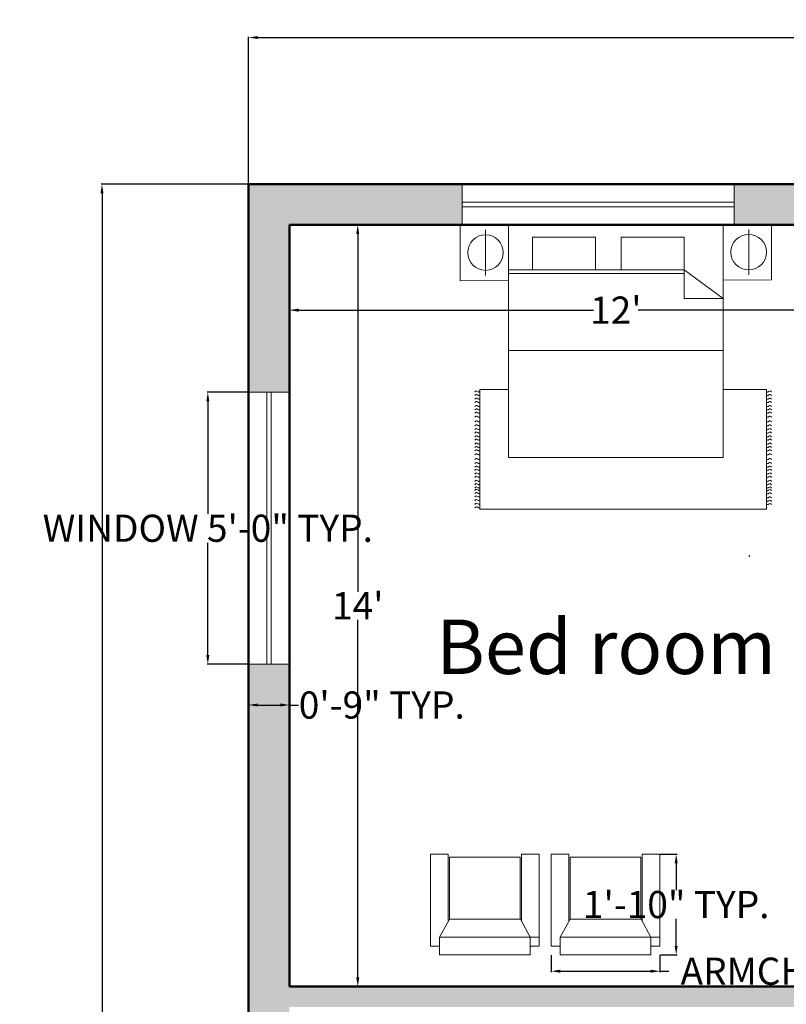
# Model space of a CAD drawing. Units: inches. Extents: x 2436 to 2989, y 5527 to 6207.
# Tile 3 of 5: x 2436 to 2605, y 5989 to 6207. Entities that reach past the tile are written whole.
import ezdxf

# ---------------------------------------------------------------- set-up
doc = ezdxf.new("R2010")
doc.units = ezdxf.units.IN
doc.header["$MEASUREMENT"] = 0
for name, color, linetype, lineweight in [('A-ANNO-DIMS', 2, 'Continuous', 18), ('A-AREA-IDEN', 7, 'Continuous', 25), ('A-FURN', 8, 'Continuous', 18), ('A-GLAZ', 4, 'Continuous', 18), ('A-WALL', 7, 'Continuous', 50), ('A-WALL-PATT', 252, 'Continuous', 13)]:
    doc.layers.add(name, color=color, linetype=linetype, lineweight=lineweight)
doc.styles.get("Standard").update_dxf_attribs({"font": 'arial.ttf'})
doc.dimstyles.get("Standard").update_dxf_attribs({"dimtxt": 6, "dimasz": 2, "dimexe": 0.18, "dimexo": 0.0625, "dimgap": 0.09, "dimtad": 0, "dimtih": 1, "dimtoh": 1, "dimdec": 0, "dimzin": 0, "dimdsep": 46, "dimlunit": 3, "dimtxsty": 'Standard', "dimcen": 0.09, "dimadec": 0, "dimazin": 0, "dimtfac": 1, "dimtdec": 0, "dimtofl": 0, "dimtmove": 0, "dimatfit": 3, "dimfxl": 1, "dimtolj": 1, "dimtzin": 0, "dimarcsym": 0})

# ---------------------------------------------------------------- blocks, each defined once
blk = doc.blocks.new('*D3')
at = {"layer": 'A-ANNO-DIMS', "color": 0, "lineweight": -2, "transparency": 16777216}
for p, q in [((2495.45, 6161.23), (2510.64, 6161.23)), ((2510.46, 6159.23), (2510.46, 6080.33)), ((2510.46, 5995.23), (2510.46, 6074.13)), ((2495.45, 5993.23), (2510.64, 5993.23))]:
    blk.add_line(p, q, dxfattribs=at)
at = {"layer": 'A-ANNO-DIMS', "color": 0, "transparency": 16777216}
for points in [[(2510.12, 6159.23), (2510.79, 6159.23), (2510.46, 6161.23)], [(2510.12, 5995.23), (2510.79, 5995.23), (2510.46, 5993.23)]]:
    blk.add_solid(points, dxfattribs=at)
at = {"layer": 'Defpoints', "color": 0, "transparency": 16777216}
for p in [(2495.39, 6161.23), (2495.39, 5993.23), (2510.46, 5993.23)]:
    blk.add_point(p, dxfattribs=at)
at = {"layer": 'A-ANNO-DIMS', "color": 0, "transparency": 16777216, "insert": (2510.46, 6077.23), "char_height": 6, "attachment_point": 5}
blk.add_mtext("\\A1;14'", dxfattribs=at)
blk = doc.blocks.new('*D4')
at = {"layer": 'A-ANNO-DIMS', "color": 0, "lineweight": -2, "transparency": 16777216}
for p, q in [((2495.39, 6161.17), (2495.39, 6142.26)), ((2639.39, 6161.17), (2639.39, 6142.26)), ((2497.39, 6142.44), (2562.49, 6142.44)), ((2637.39, 6142.44), (2572.29, 6142.44))]:
    blk.add_line(p, q, dxfattribs=at)
at = {"layer": 'A-ANNO-DIMS', "color": 0, "transparency": 16777216}
for points in [[(2497.39, 6142.77), (2497.39, 6142.1), (2495.39, 6142.44)], [(2637.39, 6142.77), (2637.39, 6142.1), (2639.39, 6142.44)]]:
    blk.add_solid(points, dxfattribs=at)
at = {"layer": 'Defpoints', "color": 0, "transparency": 16777216}
for p in [(2495.39, 6161.23), (2639.39, 6161.23), (2639.39, 6142.44)]:
    blk.add_point(p, dxfattribs=at)
at = {"layer": 'A-ANNO-DIMS', "color": 0, "transparency": 16777216, "insert": (2567.39, 6142.44), "char_height": 6, "attachment_point": 5}
blk.add_mtext("\\A1;12'", dxfattribs=at)
blk = doc.blocks.new('BED-WITH-NIGHTSTANDS')
for p, q in [((5.6, 61.62), (5.6, 51.56)), ((63.65, 61.72), (63.65, 51.66)), ((49.39, 52.82), (10.63, 52.82)), ((49.39, 52.82), (58, 46.47)), ((49.44, 52.82), (49.44, 46.47)), ((49.44, 52), (10.63, 52)), ((49.44, 46.47), (58, 46.47)), ((58.05, 34.96), (10.63, 34.96)), ((4.35, 0), (4.35, 26.37)), ((4.35, 26.37), (10.65, 26.37)), ((58.05, 26.37), (67.59, 26.37)), ((67.59, 26.37), (67.59, 0)), ((4.35, 0), (67.59, 0))]:
    blk.add_line(p, q)
for points in [[(0, 50.39), (10.63, 50.5), (10.63, 62.68), (0, 62.58)], [(58.05, 62.68), (58.05, 11.37), (10.63, 11.37), (10.63, 62.68)], [(58.05, 50.5), (68.68, 50.6), (68.68, 62.78), (58.05, 62.68)], [(29.88, 59.98), (29.88, 52.82), (15.98, 52.82), (15.98, 59.98)], [(49.44, 59.98), (49.44, 52.82), (35.55, 52.82), (35.55, 59.98)]]:
    blk.add_lwpolyline(points, close=True)
for centre in [(5.6, 56.59), (63.65, 56.69)]:
    blk.add_circle(centre, 3.92)
for points, knots in [([(3.23, 25.84), (3.32, 25.96), (3.52, 26.2), (3.86, 25.96), (4.14, 25.78), (4.29, 25.89), (4.35, 25.94)], [0, 0, 0, 0, 0.400747, 0.791423, 1.067667, 1.29709, 1.29709, 1.29709, 1.29709]), ([(68.71, 25.84), (68.61, 25.96), (68.42, 26.2), (68.08, 25.96), (67.8, 25.78), (67.65, 25.89), (67.58, 25.94)], [0, 0, 0, 0, 0.400747, 0.791423, 1.067667, 1.29709, 1.29709, 1.29709, 1.29709]), ([(3.23, 25.06), (3.32, 25.18), (3.52, 25.42), (3.86, 25.18), (4.14, 25.01), (4.29, 25.11), (4.35, 25.16)], [0, 0, 0, 0, 0.400747, 0.791423, 1.067667, 1.29709, 1.29709, 1.29709, 1.29709]), ([(3.23, 24.24), (3.32, 24.36), (3.52, 24.6), (3.86, 24.36), (4.14, 24.19), (4.29, 24.3), (4.35, 24.34)], [0, 0, 0, 0, 0.400747, 0.791423, 1.067667, 1.29709, 1.29709, 1.29709, 1.29709]), ([(68.71, 25.06), (68.61, 25.18), (68.42, 25.42), (68.08, 25.18), (67.8, 25.01), (67.65, 25.11), (67.58, 25.16)], [0, 0, 0, 0, 0.400747, 0.791423, 1.067667, 1.29709, 1.29709, 1.29709, 1.29709]), ([(68.71, 24.24), (68.61, 24.36), (68.42, 24.6), (68.08, 24.36), (67.8, 24.19), (67.65, 24.3), (67.58, 24.34)], [0, 0, 0, 0, 0.400747, 0.791423, 1.067667, 1.29709, 1.29709, 1.29709, 1.29709]), ([(3.23, 23.51), (3.32, 23.63), (3.52, 23.87), (3.86, 23.63), (4.14, 23.46), (4.29, 23.57), (4.35, 23.62)], [0, 0, 0, 0, 0.400747, 0.791423, 1.067667, 1.29709, 1.29709, 1.29709, 1.29709]), ([(3.23, 22.63), (3.32, 22.75), (3.52, 22.99), (3.86, 22.75), (4.14, 22.58), (4.29, 22.69), (4.35, 22.73)], [0, 0, 0, 0, 0.400747, 0.791423, 1.067667, 1.29709, 1.29709, 1.29709, 1.29709]), ([(3.23, 21.88), (3.32, 22), (3.52, 22.24), (3.86, 22), (4.14, 21.83), (4.29, 21.93), (4.35, 21.98)], [0, 0, 0, 0, 0.400747, 0.791423, 1.067667, 1.29709, 1.29709, 1.29709, 1.29709]), ([(68.71, 23.51), (68.61, 23.63), (68.42, 23.87), (68.08, 23.63), (67.8, 23.46), (67.65, 23.57), (67.58, 23.62)], [0, 0, 0, 0, 0.400747, 0.791423, 1.067667, 1.29709, 1.29709, 1.29709, 1.29709]), ([(68.71, 22.63), (68.61, 22.75), (68.42, 22.99), (68.08, 22.75), (67.8, 22.58), (67.65, 22.69), (67.58, 22.73)], [0, 0, 0, 0, 0.400747, 0.791423, 1.067667, 1.29709, 1.29709, 1.29709, 1.29709]), ([(68.71, 21.88), (68.61, 22), (68.42, 22.24), (68.08, 22), (67.8, 21.83), (67.65, 21.93), (67.58, 21.98)], [0, 0, 0, 0, 0.400747, 0.791423, 1.067667, 1.29709, 1.29709, 1.29709, 1.29709]), ([(3.23, 21.15), (3.32, 21.27), (3.52, 21.51), (3.86, 21.27), (4.14, 21.1), (4.29, 21.21), (4.35, 21.25)], [0, 0, 0, 0, 0.400747, 0.791423, 1.067667, 1.29709, 1.29709, 1.29709, 1.29709]), ([(3.23, 20.27), (3.32, 20.39), (3.52, 20.63), (3.86, 20.39), (4.14, 20.22), (4.29, 20.32), (4.35, 20.37)], [0, 0, 0, 0, 0.400747, 0.791423, 1.067667, 1.29709, 1.29709, 1.29709, 1.29709]), ([(68.71, 21.15), (68.61, 21.27), (68.42, 21.51), (68.08, 21.27), (67.8, 21.1), (67.65, 21.21), (67.58, 21.25)], [0, 0, 0, 0, 0.400747, 0.791423, 1.067667, 1.29709, 1.29709, 1.29709, 1.29709]), ([(68.71, 20.27), (68.61, 20.39), (68.42, 20.63), (68.08, 20.39), (67.8, 20.22), (67.65, 20.32), (67.58, 20.37)], [0, 0, 0, 0, 0.400747, 0.791423, 1.067667, 1.29709, 1.29709, 1.29709, 1.29709]), ([(3.23, 19.23), (3.32, 19.35), (3.52, 19.59), (3.86, 19.35), (4.14, 19.18), (4.29, 19.29), (4.35, 19.33)], [0, 0, 0, 0, 0.400747, 0.791423, 1.067667, 1.29709, 1.29709, 1.29709, 1.29709]), ([(3.23, 18.35), (3.32, 18.47), (3.52, 18.71), (3.86, 18.47), (4.14, 18.3), (4.29, 18.4), (4.35, 18.45)], [0, 0, 0, 0, 0.400747, 0.791423, 1.067667, 1.29709, 1.29709, 1.29709, 1.29709]), ([(3.23, 17.53), (3.32, 17.65), (3.52, 17.89), (3.86, 17.65), (4.14, 17.48), (4.29, 17.59), (4.35, 17.64)], [0, 0, 0, 0, 0.400747, 0.791423, 1.067667, 1.29709, 1.29709, 1.29709, 1.29709]), ([(68.71, 19.23), (68.61, 19.35), (68.42, 19.59), (68.08, 19.35), (67.8, 19.18), (67.65, 19.29), (67.58, 19.33)], [0, 0, 0, 0, 0.400747, 0.791423, 1.067667, 1.29709, 1.29709, 1.29709, 1.29709]), ([(68.71, 18.35), (68.61, 18.47), (68.42, 18.71), (68.08, 18.47), (67.8, 18.3), (67.65, 18.4), (67.58, 18.45)], [0, 0, 0, 0, 0.400747, 0.791423, 1.067667, 1.29709, 1.29709, 1.29709, 1.29709]), ([(68.71, 17.53), (68.61, 17.65), (68.42, 17.89), (68.08, 17.65), (67.8, 17.48), (67.65, 17.59), (67.58, 17.64)], [0, 0, 0, 0, 0.400747, 0.791423, 1.067667, 1.29709, 1.29709, 1.29709, 1.29709]), ([(3.23, 16.76), (3.32, 16.88), (3.52, 17.12), (3.86, 16.88), (4.14, 16.71), (4.29, 16.81), (4.35, 16.86)], [0, 0, 0, 0, 0.400747, 0.791423, 1.067667, 1.29709, 1.29709, 1.29709, 1.29709]), ([(3.23, 15.94), (3.32, 16.06), (3.52, 16.3), (3.86, 16.06), (4.14, 15.89), (4.29, 16), (4.35, 16.04)], [0, 0, 0, 0, 0.400747, 0.791423, 1.067667, 1.29709, 1.29709, 1.29709, 1.29709]), ([(3.23, 15.21), (3.32, 15.33), (3.52, 15.57), (3.86, 15.33), (4.14, 15.16), (4.29, 15.27), (4.35, 15.32)], [0, 0, 0, 0, 0.400747, 0.791423, 1.067667, 1.29709, 1.29709, 1.29709, 1.29709]), ([(68.71, 16.76), (68.61, 16.88), (68.42, 17.12), (68.08, 16.88), (67.8, 16.71), (67.65, 16.81), (67.58, 16.86)], [0, 0, 0, 0, 0.400747, 0.791423, 1.067667, 1.29709, 1.29709, 1.29709, 1.29709]), ([(68.71, 15.94), (68.61, 16.06), (68.42, 16.3), (68.08, 16.06), (67.8, 15.89), (67.65, 16), (67.58, 16.04)], [0, 0, 0, 0, 0.400747, 0.791423, 1.067667, 1.29709, 1.29709, 1.29709, 1.29709]), ([(68.71, 15.21), (68.61, 15.33), (68.42, 15.57), (68.08, 15.33), (67.8, 15.16), (67.65, 15.27), (67.58, 15.32)], [0, 0, 0, 0, 0.400747, 0.791423, 1.067667, 1.29709, 1.29709, 1.29709, 1.29709]), ([(3.23, 14.33), (3.32, 14.45), (3.52, 14.69), (3.86, 14.45), (4.14, 14.28), (4.29, 14.39), (4.35, 14.43)], [0, 0, 0, 0, 0.400747, 0.791423, 1.067667, 1.29709, 1.29709, 1.29709, 1.29709]), ([(3.23, 13.58), (3.32, 13.7), (3.52, 13.94), (3.86, 13.7), (4.14, 13.53), (4.29, 13.63), (4.35, 13.68)], [0, 0, 0, 0, 0.400747, 0.791423, 1.067667, 1.29709, 1.29709, 1.29709, 1.29709]), ([(3.23, 12.85), (3.32, 12.97), (3.52, 13.21), (3.86, 12.97), (4.14, 12.8), (4.29, 12.9), (4.35, 12.95)], [0, 0, 0, 0, 0.400747, 0.791423, 1.067667, 1.29709, 1.29709, 1.29709, 1.29709]), ([(68.71, 14.33), (68.61, 14.45), (68.42, 14.69), (68.08, 14.45), (67.8, 14.28), (67.65, 14.39), (67.58, 14.43)], [0, 0, 0, 0, 0.400747, 0.791423, 1.067667, 1.29709, 1.29709, 1.29709, 1.29709]), ([(68.71, 13.58), (68.61, 13.7), (68.42, 13.94), (68.08, 13.7), (67.8, 13.53), (67.65, 13.63), (67.58, 13.68)], [0, 0, 0, 0, 0.400747, 0.791423, 1.067667, 1.29709, 1.29709, 1.29709, 1.29709]), ([(68.71, 12.85), (68.61, 12.97), (68.42, 13.21), (68.08, 12.97), (67.8, 12.8), (67.65, 12.9), (67.58, 12.95)], [0, 0, 0, 0, 0.400747, 0.791423, 1.067667, 1.29709, 1.29709, 1.29709, 1.29709]), ([(3.23, 11.97), (3.32, 12.09), (3.52, 12.33), (3.86, 12.09), (4.14, 11.92), (4.29, 12.02), (4.35, 12.07)], [0, 0, 0, 0, 0.400747, 0.791423, 1.067667, 1.29709, 1.29709, 1.29709, 1.29709]), ([(3.23, 10.93), (3.32, 11.05), (3.52, 11.29), (3.86, 11.05), (4.14, 10.88), (4.29, 10.99), (4.35, 11.03)], [0, 0, 0, 0, 0.400747, 0.791423, 1.067667, 1.29709, 1.29709, 1.29709, 1.29709]), ([(68.71, 11.97), (68.61, 12.09), (68.42, 12.33), (68.08, 12.09), (67.8, 11.92), (67.65, 12.02), (67.58, 12.07)], [0, 0, 0, 0, 0.400747, 0.791423, 1.067667, 1.29709, 1.29709, 1.29709, 1.29709]), ([(68.71, 10.93), (68.61, 11.05), (68.42, 11.29), (68.08, 11.05), (67.8, 10.88), (67.65, 10.99), (67.58, 11.03)], [0, 0, 0, 0, 0.400747, 0.791423, 1.067667, 1.29709, 1.29709, 1.29709, 1.29709]), ([(3.23, 10.05), (3.32, 10.17), (3.52, 10.41), (3.86, 10.17), (4.14, 10), (4.29, 10.1), (4.35, 10.15)], [0, 0, 0, 0, 0.400747, 0.791423, 1.067667, 1.29709, 1.29709, 1.29709, 1.29709]), ([(3.23, 9.23), (3.32, 9.35), (3.52, 9.59), (3.86, 9.35), (4.14, 9.18), (4.29, 9.29), (4.35, 9.34)], [0, 0, 0, 0, 0.400747, 0.791423, 1.067667, 1.29709, 1.29709, 1.29709, 1.29709]), ([(3.23, 8.54), (3.32, 8.66), (3.52, 8.9), (3.86, 8.66), (4.14, 8.49), (4.29, 8.6), (4.35, 8.65)], [0, 0, 0, 0, 0.400747, 0.791423, 1.067667, 1.29709, 1.29709, 1.29709, 1.29709]), ([(68.71, 10.05), (68.61, 10.17), (68.42, 10.41), (68.08, 10.17), (67.8, 10), (67.65, 10.1), (67.58, 10.15)], [0, 0, 0, 0, 0.400747, 0.791423, 1.067667, 1.29709, 1.29709, 1.29709, 1.29709]), ([(68.71, 9.23), (68.61, 9.35), (68.42, 9.59), (68.08, 9.35), (67.8, 9.18), (67.65, 9.29), (67.58, 9.34)], [0, 0, 0, 0, 0.400747, 0.791423, 1.067667, 1.29709, 1.29709, 1.29709, 1.29709]), ([(68.71, 8.54), (68.61, 8.66), (68.42, 8.9), (68.08, 8.66), (67.8, 8.49), (67.65, 8.6), (67.58, 8.65)], [0, 0, 0, 0, 0.400747, 0.791423, 1.067667, 1.29709, 1.29709, 1.29709, 1.29709]), ([(3.23, 7.73), (3.32, 7.85), (3.52, 8.09), (3.86, 7.85), (4.14, 7.68), (4.29, 7.78), (4.35, 7.83)], [0, 0, 0, 0, 0.400747, 0.791423, 1.067667, 1.29709, 1.29709, 1.29709, 1.29709]), ([(3.23, 7), (3.32, 7.12), (3.52, 7.36), (3.86, 7.12), (4.14, 6.95), (4.29, 7.05), (4.35, 7.1)], [0, 0, 0, 0, 0.400747, 0.791423, 1.067667, 1.29709, 1.29709, 1.29709, 1.29709]), ([(68.71, 7.73), (68.61, 7.85), (68.42, 8.09), (68.08, 7.85), (67.8, 7.68), (67.65, 7.78), (67.58, 7.83)], [0, 0, 0, 0, 0.400747, 0.791423, 1.067667, 1.29709, 1.29709, 1.29709, 1.29709]), ([(68.71, 7), (68.61, 7.12), (68.42, 7.36), (68.08, 7.12), (67.8, 6.95), (67.65, 7.05), (67.58, 7.1)], [0, 0, 0, 0, 0.400747, 0.791423, 1.067667, 1.29709, 1.29709, 1.29709, 1.29709]), ([(3.23, 6.12), (3.32, 6.24), (3.52, 6.48), (3.86, 6.24), (4.14, 6.07), (4.29, 6.17), (4.35, 6.22)], [0, 0, 0, 0, 0.400747, 0.791423, 1.067667, 1.29709, 1.29709, 1.29709, 1.29709]), ([(3.23, 5.36), (3.32, 5.49), (3.52, 5.73), (3.86, 5.49), (4.14, 5.31), (4.29, 5.42), (4.35, 5.47)], [0, 0, 0, 0, 0.400747, 0.791423, 1.067667, 1.29709, 1.29709, 1.29709, 1.29709]), ([(3.23, 4.64), (3.32, 4.76), (3.52, 5), (3.86, 4.76), (4.14, 4.59), (4.29, 4.69), (4.35, 4.74)], [0, 0, 0, 0, 0.400747, 0.791423, 1.067667, 1.29709, 1.29709, 1.29709, 1.29709]), ([(3.23, 4.13), (3.32, 4.25), (3.52, 4.49), (3.86, 4.25), (4.14, 4.08), (4.29, 4.18), (4.35, 4.23)], [0, 0, 0, 0, 0.400747, 0.791423, 1.067667, 1.29709, 1.29709, 1.29709, 1.29709]), ([(68.71, 6.12), (68.61, 6.24), (68.42, 6.48), (68.08, 6.24), (67.8, 6.07), (67.65, 6.17), (67.58, 6.22)], [0, 0, 0, 0, 0.400747, 0.791423, 1.067667, 1.29709, 1.29709, 1.29709, 1.29709]), ([(68.71, 5.36), (68.61, 5.49), (68.42, 5.73), (68.08, 5.49), (67.8, 5.31), (67.65, 5.42), (67.58, 5.47)], [0, 0, 0, 0, 0.400747, 0.791423, 1.067667, 1.29709, 1.29709, 1.29709, 1.29709]), ([(68.71, 4.64), (68.61, 4.76), (68.42, 5), (68.08, 4.76), (67.8, 4.59), (67.66, 4.69), (67.59, 4.73)], [0, 0, 0, 0, 0.400747, 0.791423, 1.067667, 1.283686, 1.283686, 1.283686, 1.283686]), ([(3.23, 3.44), (3.32, 3.56), (3.52, 3.8), (3.86, 3.56), (4.14, 3.39), (4.29, 3.49), (4.35, 3.54)], [0, 0, 0, 0, 0.400747, 0.791423, 1.067667, 1.29709, 1.29709, 1.29709, 1.29709]), ([(3.23, 2.67), (3.32, 2.79), (3.52, 3.03), (3.86, 2.79), (4.14, 2.62), (4.29, 2.73), (4.35, 2.78)], [0, 0, 0, 0, 0.400747, 0.791423, 1.067667, 1.29709, 1.29709, 1.29709, 1.29709]), ([(68.72, 4.07), (68.62, 4.19), (68.43, 4.43), (68.09, 4.19), (67.81, 4.01), (67.66, 4.12), (67.59, 4.17)], [0, 0, 0, 0, 0.400747, 0.791423, 1.067667, 1.29709, 1.29709, 1.29709, 1.29709]), ([(68.72, 3.34), (68.62, 3.46), (68.43, 3.7), (68.09, 3.46), (67.81, 3.29), (67.66, 3.39), (67.59, 3.44)], [0, 0, 0, 0, 0.400747, 0.791423, 1.067667, 1.29709, 1.29709, 1.29709, 1.29709]), ([(68.72, 2.46), (68.62, 2.58), (68.43, 2.82), (68.09, 2.58), (67.81, 2.4), (67.66, 2.51), (67.59, 2.56)], [0, 0, 0, 0, 0.400747, 0.791423, 1.067667, 1.29709, 1.29709, 1.29709, 1.29709]), ([(3.23, 1.86), (3.32, 1.98), (3.52, 2.22), (3.86, 1.98), (4.14, 1.81), (4.29, 1.92), (4.35, 1.97)], [0, 0, 0, 0, 0.400747, 0.791423, 1.067667, 1.29709, 1.29709, 1.29709, 1.29709]), ([(3.23, 1.05), (3.32, 1.17), (3.52, 1.41), (3.86, 1.17), (4.14, 1), (4.29, 1.11), (4.35, 1.15)], [0, 0, 0, 0, 0.400747, 0.791423, 1.067667, 1.29709, 1.29709, 1.29709, 1.29709]), ([(3.23, 0.28), (3.32, 0.4), (3.52, 0.64), (3.86, 0.4), (4.14, 0.22), (4.29, 0.33), (4.35, 0.38)], [0, 0, 0, 0, 0.400747, 0.791423, 1.067667, 1.29709, 1.29709, 1.29709, 1.29709]), ([(68.72, 1.7), (68.62, 1.82), (68.43, 2.06), (68.09, 1.82), (67.81, 1.65), (67.66, 1.76), (67.59, 1.81)], [0, 0, 0, 0, 0.400747, 0.791423, 1.067667, 1.29709, 1.29709, 1.29709, 1.29709]), ([(68.72, 0.98), (68.62, 1.1), (68.43, 1.34), (68.09, 1.1), (67.81, 0.93), (67.67, 1.03), (67.6, 1.07)], [0, 0, 0, 0, 0.400747, 0.791423, 1.067667, 1.283686, 1.283686, 1.283686, 1.283686])]:
    blk.add_open_spline(points, degree=3, knots=knots)
blk = doc.blocks.new('CHAIR-ARM')
for p, q in [((0, 1.96), (0, 22.23)), ((3.92, 22.23), (0, 22.23)), ((3.92, 7.54), (3.92, 22.23)), ((20.05, 7.41), (20.05, 22.23)), ((20.05, 22.23), (23.98, 22.23)), ((23.98, 1.96), (23.98, 22.23)), ((19.74, 21.58), (19.74, 7.85)), ((1.96, 3.92), (4.17, 7.85)), ((19.81, 7.85), (22.01, 3.92)), ((1.96, 3.92), (23.98, 3.92)), ((1.96, 3.92), (1.96, 0)), ((22.01, 3.92), (22.01, 0)), ((0, 1.96), (1.96, 1.96)), ((1.96, 0), (22.01, 0)), ((22.01, 1.96), (23.98, 1.96))]:
    blk.add_line(p, q)
blk.add_lwpolyline([(19.74, 21.58), (4.17, 21.58), (4.17, 7.85), (19.81, 7.85)])
blk = doc.blocks.new('WINDOW-60IN')
for p, q in [((0, 9), (0, 0)), ((60, 9), (0, 9)), ((60, 0), (60, 9)), ((60, 5), (0, 5)), ((0, 4), (60, 4)), ((0, 0), (60, 0))]:
    blk.add_line(p, q)
blk = doc.blocks.new('*D34')
at = {"layer": 'A-ANNO-DIMS', "color": 0, "lineweight": -2, "transparency": 16777216}
for p, q in [((2553.14, 6000.14), (2553.14, 5996.42)), ((2577.11, 6000.14), (2577.11, 5996.42)), ((2555.14, 5996.6), (2575.11, 5996.6)), ((2577.11, 5996.6), (2579.11, 5996.6))]:
    blk.add_line(p, q, dxfattribs=at)
at = {"layer": 'A-ANNO-DIMS', "color": 0, "transparency": 16777216}
for points in [[(2555.14, 5996.94), (2555.14, 5996.27), (2553.14, 5996.6)], [(2575.11, 5996.94), (2575.11, 5996.27), (2577.11, 5996.6)]]:
    blk.add_solid(points, dxfattribs=at)
at = {"layer": 'Defpoints', "color": 0, "transparency": 16777216}
for p in [(2553.14, 6000.2), (2577.11, 6000.2), (2577.11, 5996.6)]:
    blk.add_point(p, dxfattribs=at)
at = {"layer": 'A-ANNO-DIMS', "color": 0, "transparency": 16777216, "insert": (2621.18, 5996.6), "char_height": 6, "attachment_point": 5}
blk.add_mtext('\\A1;ARMCHAIR 2\'-0" TYP.', dxfattribs=at)
blk = doc.blocks.new('*D35')
at = {"layer": 'A-ANNO-DIMS', "color": 0, "lineweight": -2, "transparency": 16777216}
for p, q in [((2577.17, 6022.43), (2580.89, 6022.43)), ((2580.71, 6020.43), (2580.71, 6014.47)), ((2580.71, 6002.2), (2580.71, 6008.16)), ((2577.17, 6000.2), (2580.89, 6000.2))]:
    blk.add_line(p, q, dxfattribs=at)
at = {"layer": 'A-ANNO-DIMS', "color": 0, "transparency": 16777216}
for points in [[(2580.37, 6020.43), (2581.04, 6020.43), (2580.71, 6022.43)], [(2580.37, 6002.2), (2581.04, 6002.2), (2580.71, 6000.2)]]:
    blk.add_solid(points, dxfattribs=at)
at = {"layer": 'Defpoints', "color": 0, "transparency": 16777216}
for p in [(2577.11, 6022.43), (2580.71, 6022.43), (2577.11, 6000.2)]:
    blk.add_point(p, dxfattribs=at)
at = {"layer": 'A-ANNO-DIMS', "color": 0, "transparency": 16777216, "insert": (2580.71, 6011.31), "char_height": 6, "attachment_point": 5}
blk.add_mtext('\\A1;1\'-10" TYP.', dxfattribs=at)
blk = doc.blocks.new('*D38')
at = {"layer": 'A-ANNO-DIMS', "color": 0, "lineweight": -2, "transparency": 16777216}
for p, q in [((2486.33, 6124.33), (2477.21, 6124.33)), ((2477.39, 6122.33), (2477.39, 6097.53)), ((2477.39, 6066.33), (2477.39, 6091.14)), ((2486.33, 6064.33), (2477.21, 6064.33))]:
    blk.add_line(p, q, dxfattribs=at)
at = {"layer": 'A-ANNO-DIMS', "color": 0, "transparency": 16777216}
for points in [[(2477.05, 6122.33), (2477.72, 6122.33), (2477.39, 6124.33)], [(2477.05, 6066.33), (2477.72, 6066.33), (2477.39, 6064.33)]]:
    blk.add_solid(points, dxfattribs=at)
at = {"layer": 'Defpoints', "color": 0, "transparency": 16777216}
for p in [(2486.39, 6124.33), (2477.39, 6064.33), (2486.39, 6064.33)]:
    blk.add_point(p, dxfattribs=at)
at = {"layer": 'A-ANNO-DIMS', "color": 0, "transparency": 16777216, "insert": (2477.39, 6094.33), "char_height": 6, "attachment_point": 5}
blk.add_mtext('\\A1;WINDOW 5\'-0" TYP.', dxfattribs=at)
blk = doc.blocks.new('*D39')
at = {"layer": 'A-ANNO-DIMS', "color": 0, "lineweight": -2, "transparency": 16777216}
for p, q in [((2486.39, 6064.27), (2486.39, 6055.15)), ((2495.39, 6064.27), (2495.39, 6055.15)), ((2488.39, 6055.33), (2493.39, 6055.33)), ((2495.39, 6055.33), (2497.39, 6055.33))]:
    blk.add_line(p, q, dxfattribs=at)
at = {"layer": 'A-ANNO-DIMS', "color": 0, "transparency": 16777216}
for points in [[(2488.39, 6055.67), (2488.39, 6055), (2486.39, 6055.33)], [(2493.39, 6055.67), (2493.39, 6055), (2495.39, 6055.33)]]:
    blk.add_solid(points, dxfattribs=at)
at = {"layer": 'Defpoints', "color": 0, "transparency": 16777216}
for p in [(2486.39, 6064.33), (2495.39, 6064.33), (2495.39, 6055.33)]:
    blk.add_point(p, dxfattribs=at)
at = {"layer": 'A-ANNO-DIMS', "color": 0, "transparency": 16777216, "insert": (2515.76, 6055.33), "char_height": 6, "attachment_point": 5}
blk.add_mtext('\\A1;0\'-9" TYP.', dxfattribs=at)
blk = doc.blocks.new('*D48')
at = {"layer": 'A-ANNO-DIMS', "color": 0, "lineweight": -2, "transparency": 16777216}
for p, q in [((2486.39, 6170.29), (2486.39, 6202.76)), ((2488.39, 6202.58), (2705.49, 6202.58)), ((2943.39, 6202.58), (2726.28, 6202.58)), ((2945.39, 6080.73), (2945.39, 6202.76))]:
    blk.add_line(p, q, dxfattribs=at)
at = {"layer": 'A-ANNO-DIMS', "color": 0, "transparency": 16777216}
for points in [[(2488.39, 6202.92), (2488.39, 6202.25), (2486.39, 6202.58)], [(2943.39, 6202.92), (2943.39, 6202.25), (2945.39, 6202.58)]]:
    blk.add_solid(points, dxfattribs=at)
at = {"layer": 'Defpoints', "color": 0, "transparency": 16777216}
for p in [(2945.39, 6202.58), (2486.39, 6170.23), (2945.39, 6080.66)]:
    blk.add_point(p, dxfattribs=at)
at = {"layer": 'A-ANNO-DIMS', "color": 0, "transparency": 16777216, "insert": (2715.89, 6202.58), "char_height": 6, "attachment_point": 5}
blk.add_mtext('\\A1;38\'-3"', dxfattribs=at)
blk = doc.blocks.new('*D49')
at = {"layer": 'A-ANNO-DIMS', "color": 0, "lineweight": -2, "transparency": 16777216}
for p, q in [((2486.33, 6170.23), (2453.86, 6170.23)), ((2454.04, 6168.23), (2454.04, 5851.68)), ((2454.04, 5528.73), (2454.04, 5845.29)), ((2675.33, 5526.73), (2453.86, 5526.73))]:
    blk.add_line(p, q, dxfattribs=at)
at = {"layer": 'A-ANNO-DIMS', "color": 0, "transparency": 16777216}
for points in [[(2453.7, 6168.23), (2454.37, 6168.23), (2454.04, 6170.23)], [(2453.7, 5528.73), (2454.37, 5528.73), (2454.04, 5526.73)]]:
    blk.add_solid(points, dxfattribs=at)
at = {"layer": 'Defpoints', "color": 0, "transparency": 16777216}
for p in [(2486.39, 6170.23), (2454.04, 5526.73), (2675.39, 5526.73)]:
    blk.add_point(p, dxfattribs=at)
at = {"layer": 'A-ANNO-DIMS', "color": 0, "transparency": 16777216, "insert": (2454.04, 5848.48), "char_height": 6, "attachment_point": 5}
blk.add_mtext('\\A1;53\'-7 1/2"', dxfattribs=at)
blk = doc.blocks.new('*D56')
at = {"layer": 'A-ANNO-DIMS', "color": 0, "lineweight": -2, "transparency": 16777216}
for p, q in [((2596.78, 6088.19), (2596.96, 6088.19)), ((2596.87, 6088.1), (2596.87, 6088.28)), ((2699.31, 6088.19), (2662.89, 6088.19))]:
    blk.add_line(p, q, dxfattribs=at)
at = {"layer": 'A-ANNO-DIMS', "color": 0, "transparency": 16777216}
blk.add_solid([(2662.89, 6088.52), (2662.89, 6087.85), (2660.89, 6088.19)], dxfattribs=at)
at = {"layer": 'Defpoints', "color": 0, "transparency": 16777216}
for p in [(2596.87, 6088.19), (2660.89, 6088.19)]:
    blk.add_point(p, dxfattribs=at)
at = {"layer": 'A-ANNO-DIMS', "color": 0, "transparency": 16777216, "insert": (2716.81, 6088.19), "char_height": 6, "attachment_point": 5}
blk.add_mtext('\\A1;4X R5\'-4"', dxfattribs=at)

msp = doc.modelspace()

# ---------------------------------------------------------------- hatches: boundary and pattern name
at = {"layer": 'A-WALL-PATT'}
h = msp.add_hatch(color=256, dxfattribs=at)
h.dxf.hatch_style = 1
h.paths.add_polyline_path([(2533.49, 6170.23), (2486.39, 6170.23), (2486.39, 6124.33), (2495.39, 6124.33), (2495.39, 6161.23), (2533.49, 6161.23)])
h.paths.add_polyline_path([(2677.58, 6170.23), (2593.49, 6170.23), (2593.49, 6161.23), (2639.39, 6161.23), (2639.39, 6035.73), (2639.39, 6035.73), (2643.89, 6035.73), (2643.89, 6036.73), (2685.89, 6036.73), (2685.89, 6041.23), (2643.89, 6041.23), (2643.89, 6161.23), (2677.58, 6161.23)])
h.paths.add_polyline_path([(2792.39, 6170.23), (2737.58, 6170.23), (2737.58, 6161.23), (2787.89, 6161.23), (2787.89, 6084.23), (2792.39, 6084.23), (2792.39, 6161.23), (2936.39, 6161.23), (2936.39, 6071.23), (2840.39, 6071.23), (2840.39, 6047.23), (2792.39, 6047.23), (2792.39, 6048.23), (2787.89, 6048.23), (2787.89, 6047.23), (2787.89, 6041.23), (2742.3, 6041.23), (2742.3, 6036.73), (2787.89, 6036.73), (2787.89, 6035.73), (2792.39, 6035.73), (2792.39, 6042.73), (2840.39, 6042.73), (2840.39, 5945.23), (2792.39, 5945.23), (2792.39, 6003.73), (2787.89, 6003.73), (2787.89, 5893.73), (2792.39, 5893.73), (2792.39, 5940.73), (2845.89, 5940.73), (2845.89, 5945.23), (2844.89, 5945.23), (2844.89, 6047.23), (2844.89, 6066.73), (2936.39, 6066.73), (2936.39, 6024.33), (2945.39, 6024.33), (2945.39, 6080.66), (2940.89, 6080.66), (2940.89, 6165.73), (2792.39, 6165.73)])
h.paths.add_polyline_path([(2945.39, 6000.33), (2936.39, 6000.33), (2936.39, 5945.23), (2881.89, 5945.23), (2881.89, 5940.73), (2936.39, 5940.73), (2936.39, 5901.74), (2945.39, 5901.74)], flags=17)
h.paths.add_polyline_path([(2945.39, 5841.74), (2936.39, 5841.74), (2936.39, 5796.73), (2792.39, 5796.73), (2792.39, 5857.73), (2787.89, 5857.73), (2787.89, 5856.73), (2786.89, 5856.73), (2786.89, 5852.23), (2787.89, 5852.23), (2787.89, 5792.23), (2892.89, 5792.23), (2892.89, 5760.78), (2901.89, 5760.78), (2901.89, 5792.23), (2945.39, 5792.23)])
h.paths.add_polyline_path([(2495.39, 5880.74), (2486.39, 5880.74), (2486.39, 5787.73), (2525.39, 5787.73), (2525.39, 5761.57), (2534.39, 5761.57), (2534.39, 5792.23), (2639.39, 5792.23), (2639.39, 5733.23), (2643.89, 5733.23), (2643.89, 5852.23), (2750.89, 5852.23), (2750.89, 5856.73), (2643.89, 5856.73), (2643.89, 5857.73), (2639.39, 5857.73), (2639.39, 5796.73), (2495.39, 5796.73)])
h.paths.add_polyline_path([(2495.39, 6064.33), (2486.39, 6064.33), (2486.39, 5940.74), (2495.39, 5940.74), (2495.39, 5988.73), (2639.39, 5988.73), (2639.39, 5893.73), (2643.89, 5893.73), (2643.89, 5999.73), (2639.39, 5999.73), (2639.39, 5993.23), (2495.39, 5993.23)])
h.paths.add_polyline_path([(2682.14, 5696.23), (2643.89, 5696.23), (2643.89, 5697.23), (2639.39, 5697.23), (2639.39, 5696.23), (2558.39, 5696.23), (2534.39, 5696.23), (2534.39, 5737.57), (2525.39, 5737.57), (2525.39, 5687.23), (2534.39, 5687.23), (2558.39, 5687.23), (2643.89, 5687.23), (2682.14, 5687.23)])
h.paths.add_polyline_path([(2901.89, 5736.78), (2892.89, 5736.78), (2892.89, 5696.23), (2868.89, 5696.23), (2751.89, 5696.23), (2751.89, 5687.23), (2787.89, 5687.23), (2787.89, 5567.23), (2792.39, 5567.23), (2792.39, 5687.23), (2868.89, 5687.23), (2892.89, 5687.23), (2901.89, 5687.23)])
h.paths.add_polyline_path([(2643.89, 5687.23), (2639.39, 5687.23), (2639.39, 5567.23), (2643.89, 5567.23)])
h.paths.add_polyline_path([(2787.89, 5567.23), (2643.89, 5567.23), (2643.89, 5562.73), (2787.89, 5562.73)])
h.paths.add_polyline_path([(2643.89, 5567.23), (2639.39, 5567.23), (2639.39, 5562.73), (2643.89, 5562.73)])
h.paths.add_polyline_path([(2792.39, 5567.23), (2787.89, 5567.23), (2787.89, 5562.73), (2792.39, 5562.73)])

# ---------------------------------------------------------------- linework, layer by layer
at = {"layer": 'A-GLAZ'}
msp.add_line((2533.49, 6161.23), (2533.49, 6161.23), dxfattribs=at)
at = {"layer": 'A-WALL'}
for p, q in [((2486.39, 6170.23), (2792.39, 6170.23)), ((2486.39, 6170.23), (2486.39, 5787.73)), ((2495.39, 6161.23), (2639.39, 6161.23)), ((2495.39, 6161.23), (2495.39, 5993.23)), ((2495.39, 5993.23), (2639.39, 5993.23))]:
    msp.add_line(p, q, dxfattribs=at)

# ---------------------------------------------------------------- block references
at = {"layer": 'A-FURN'}
for name, p in [('BED-WITH-NIGHTSTANDS', (2533.05, 6098.55)), ('CHAIR-ARM', (2526.52, 6000.2)), ('CHAIR-ARM', (2553.14, 6000.2))]:
    msp.add_blockref(name, p, dxfattribs=at)
at = {"layer": 'A-GLAZ'}
msp.add_blockref('WINDOW-60IN', (2533.49, 6161.23), dxfattribs=at)
at = {"layer": 'A-GLAZ', "rotation": 270.0000000000037}
msp.add_blockref('WINDOW-60IN', (2486.39, 6124.33), dxfattribs=at)

# ---------------------------------------------------------------- texts
at = {"layer": 'A-AREA-IDEN', "insert": (2527.74, 6074.17), "char_height": 12, "attachment_point": 1}
msp.add_mtext_dynamic_manual_height_columns('Bed room', width=83.0304, gutter_width=1, heights=[0], dxfattribs=at)

# ---------------------------------------------------------------- dimensions: what is measured, and where the dimension line sits
at = {"layer": 'A-ANNO-DIMS'}
for base, p1, p2, override, picture, middle in [((2945.39, 6202.58), (2486.39, 6170.23), (2945.39, 6080.66), {"dimdec": 1, "dimlfac": 1, "dimrnd": 0, "dimzin": 1, "dimdsep": 46, "dimlunit": 4, "dimfrac": 2}, '*D48', (2715.89, 6202.58)), ((2639.39, 6142.44), (2495.39, 6161.23), (2639.39, 6161.23), {"dimclrd": 0, "dimclre": 0, "dimclrt": 0}, '*D4', (2567.39, 6142.44))]:
    dim = msp.add_linear_dim(base=base, p1=p1, p2=p2, dimstyle='Standard', override=override, dxfattribs=at)
    dim.commit()
    dim.dimension.update_dxf_attribs({"geometry": picture, "text_midpoint": middle})
for base, p1, p2, override, picture, middle in [((2454.04, 5526.73), (2486.39, 6170.23), (2675.39, 5526.73), {"dimdec": 1, "dimlfac": 1, "dimrnd": 0, "dimzin": 1, "dimdsep": 46, "dimlunit": 4, "dimfrac": 2}, '*D49', (2454.04, 5848.48)), ((2510.46, 5993.23), (2495.39, 6161.23), (2495.39, 5993.23), {"dimclrd": 0, "dimclre": 0, "dimclrt": 0}, '*D3', (2510.46, 6077.23))]:
    dim = msp.add_linear_dim(base=base, p1=p1, p2=p2, angle=90, dimstyle='Standard', override=override, dxfattribs=at)
    dim.commit()
    dim.dimension.update_dxf_attribs({"geometry": picture, "text_midpoint": middle})
for base, p1, p2, angle, text, picture, middle in [((2477.39, 6064.33), (2486.39, 6124.33), (2486.39, 6064.33), 270, 'WINDOW <> TYP.', '*D38', (2477.39, 6094.33)), ((2580.71, 6022.43), (2577.11, 6000.2), (2577.11, 6022.43), 90, '<> TYP.', '*D35', (2580.71, 6011.31))]:
    dim = msp.add_linear_dim(base=base, p1=p1, p2=p2, angle=angle, text=text, dimstyle='Standard', override={"dimdec": 1, "dimlfac": 1, "dimrnd": 0, "dimzin": 1, "dimdsep": 46, "dimlunit": 4, "dimfrac": 2}, dxfattribs=at)
    dim.commit()
    dim.dimension.update_dxf_attribs({"geometry": picture, "text_midpoint": middle})
dim = msp.add_radius_dim(center=(2596.87, 6088.19), mpoint=(2660.89, 6088.19), text='4X <>', dimstyle='Standard', override={"dimdec": 1, "dimlfac": 1, "dimrnd": 0, "dimzin": 1, "dimdsep": 46, "dimlunit": 4, "dimfrac": 2}, dxfattribs=at)
dim.commit()
dim.dimension.update_dxf_attribs({"geometry": '*D56', "text_midpoint": (2699.31, 6088.19), "dimtype": 164})
for base, p1, p2, text, picture, middle in [((2495.39, 6055.33), (2486.39, 6064.33), (2495.39, 6064.33), '<> TYP.', '*D39', (2515.76, 6055.33)), ((2577.11, 5996.6), (2553.14, 6000.2), (2577.11, 6000.2), 'ARMCHAIR <> TYP.', '*D34', (2621.18, 5996.6))]:
    dim = msp.add_linear_dim(base=base, p1=p1, p2=p2, text=text, dimstyle='Standard', override={"dimdec": 1, "dimlfac": 1, "dimrnd": 0, "dimzin": 1, "dimdsep": 46, "dimlunit": 4, "dimfrac": 2}, dxfattribs=at)
    dim.commit()
    dim.dimension.update_dxf_attribs({"geometry": picture, "text_midpoint": middle})

doc.saveas('drawing.dxf')
